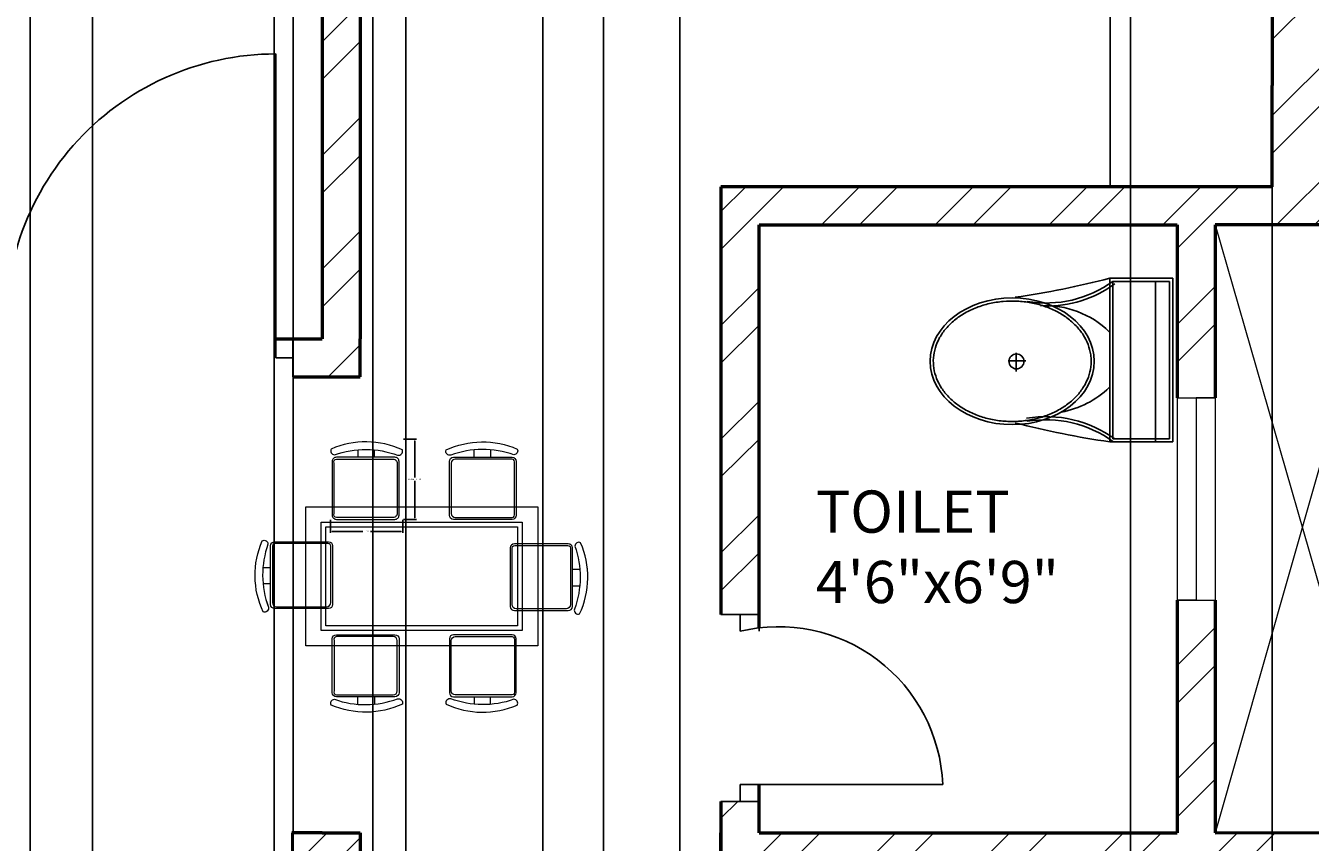
# Model space of a CAD drawing. Units: inches. Extents: x 1980 to 2738, y 1471 to 2568.
# Tile 18 of 22: x 2211 to 2363, y 2232 to 2329. Entities that reach past the tile are written whole.
import ezdxf

# ---------------------------------------------------------------- set-up
doc = ezdxf.new("R2010")
doc.units = ezdxf.units.IN
for name, color, linetype, lineweight in [('A-ANNO-DIMS', 2, 'Continuous', 18), ('A-AREA-IDEN', 7, 'Continuous', 18), ('A-DOOR', 31, 'Continuous', 25), ('A-FLOR-CASE', 8, 'Continuous', 25), ('A-FLOR-FIXT', 8, 'Continuous', 25), ('A-FLOR-OPEN', 8, 'Continuous', 18), ('A-FURN', 8, 'Continuous', 18), ('A-GLAZ', 141, 'Continuous', 18), ('A-WALL', 7, 'Continuous', 50)]:
    doc.layers.add(name, color=color, linetype=linetype, lineweight=lineweight)
doc.layers.add('A-WALL-PATT', color=9, linetype='Continuous', lineweight=13, true_color=0xd19cc7)
doc.styles.get("Standard").update_dxf_attribs({"font": 'arial.ttf'})
doc.dimstyles.get("Standard").update_dxf_attribs({"dimtxt": 0.18, "dimasz": 0.18, "dimexe": 0.18, "dimexo": 0.0625, "dimgap": 0.09, "dimtad": 0, "dimtih": 1, "dimtoh": 1, "dimdec": 4, "dimzin": 0, "dimdsep": 46, "dimtxsty": 'Standard', "dimcen": 0.09, "dimadec": 0, "dimazin": 0, "dimtfac": 1, "dimtdec": 4, "dimtofl": 0, "dimtmove": 0, "dimatfit": 3, "dimfxl": 1, "dimtolj": 1, "dimtzin": 0, "dimarcsym": 0})

# ---------------------------------------------------------------- blocks, each defined once
blk = doc.blocks.new('A$C31115884')
for p, q in [((283.1, 497.7), (223.4, 497.7)), ((257.5, 466.4), (257.5, 523.2)), ((0, 200), (0, 0)), ((520, 200), (0, 200)), ((10, 190), (10, 10)), ((510, 190), (10, 190)), ((510, 10), (510, 190)), ((520, 0), (520, 200)), ((510, 54.5), (0, 54.5)), ((10, 10), (510, 10)), ((0, 0), (520, 0))]:
    blk.add_line(p, q)
blk.add_circle((255.6, 496.4), 23.6)
for centre, radius, start, end in [((2777.7, -204.6), 2807, 165.4549, 171.7133), ((3237, 905), 2807, 188.2867, 194.5451), ((-294.5, 403.3), 364.7, 324.2091, 9.3499), ((-294.5, 403.3), 374.7, 324.2091, 9.3499), ((805.8, 403.3), 364.7, 170.6501, 215.7909), ((139.5, 406.2), 293.5, 315.8436, 2.6563), ((805.8, 403.3), 374.7, 179.2036, 215.7909), ((383.6, 406.2), 293.5, 190.2774, 224.1564)]:
    blk.add_arc(centre, radius, start, end)
blk.add_ellipse((256.2, 509.9), major_axis=(0, -260.7), ratio=0.772727)
blk.add_open_spline([(256.2, 259.2), (263.1, 259.2), (270, 259.7), (287.8, 262.3), (298.7, 265.1), (319.9, 273.1), (330.2, 278.4), (350.1, 291.1), (359.7, 298.7), (377.7, 315.9), (386.2, 325.5), (401.7, 346.6), (408.8, 358.1), (421.3, 382.5), (426.8, 395.5), (435.9, 422.4), (439.5, 436.4), (444.8, 465.1), (446.5, 479.7), (447.9, 509.2), (447.6, 524), (445, 553.3), (442.7, 567.8), (436.3, 596), (432.1, 609.7), (421.9, 636), (416, 648.6), (402.5, 672.1), (395, 683), (378.6, 703), (369.8, 712.1), (351.1, 728), (341.3, 734.8), (320.9, 746.2), (310.4, 750.7), (288.9, 757.3), (278, 759.4), (256, 761), (245, 760.6), (223.1, 757.2), (212.3, 754.3), (191.1, 746.1), (180.8, 740.7), (160.9, 727.8), (151.4, 720.1), (133.5, 702.7), (125.1, 693), (109.6, 671.7), (102.6, 660.2), (90.2, 635.7), (84.9, 622.7), (76, 595.6), (72.4, 581.6), (67.2, 552.9), (65.6, 538.2), (64.4, 508.8), (64.8, 494), (67.5, 464.7), (69.9, 450.2), (76.6, 422), (80.8, 408.3), (91.1, 382.2), (97.2, 369.7), (110.8, 346.3), (118.4, 335.4), (134.8, 315.6), (143.7, 306.7), (162.4, 290.9), (172.3, 284.2), (192.8, 273), (203.3, 268.6), (224.8, 262.2), (235.8, 260.2), (249.9, 259.3), (253, 259.2), (256.2, 259.2)], degree=3, knots=[0, 0, 0, 0, 0.110105, 0.110105, 0.285049, 0.285049, 0.459994, 0.459994, 0.634938, 0.634938, 0.809882, 0.809882, 0.984827, 0.984827, 1.159771, 1.159771, 1.334715, 1.334715, 1.50966, 1.50966, 1.684604, 1.684604, 1.859549, 1.859549, 2.034493, 2.034493, 2.209437, 2.209437, 2.384382, 2.384382, 2.559326, 2.559326, 2.73427, 2.73427, 2.909215, 2.909215, 3.084159, 3.084159, 3.259103, 3.259103, 3.434048, 3.434048, 3.608992, 3.608992, 3.783936, 3.783936, 3.958881, 3.958881, 4.133825, 4.133825, 4.30877, 4.30877, 4.483714, 4.483714, 4.658658, 4.658658, 4.833603, 4.833603, 5.008547, 5.008547, 5.183491, 5.183491, 5.358436, 5.358436, 5.53338, 5.53338, 5.708324, 5.708324, 5.883269, 5.883269, 6.058213, 6.058213, 6.233158, 6.233158, 6.283185, 6.283185, 6.283185, 6.283185])
blk = doc.blocks.new('TABLE-DINING-RECT')
for points in [[(0, 16.47), (27.45, 16.47), (27.45, 0), (0, 0)], [(0, 16.47), (27.45, 16.47), (27.45, 0), (0, 0)], [(1.83, 14.64), (25.62, 14.64), (25.62, 1.83), (1.83, 1.83)], [(1.83, 14.64), (25.62, 14.64), (25.62, 1.83), (1.83, 1.83)], [(2.38, 14.09), (25.07, 14.09), (25.07, 2.38), (2.38, 2.38)], [(2.38, 14.09), (25.07, 14.09), (25.07, 2.38), (2.38, 2.38)]]:
    blk.add_lwpolyline(points, close=True)
blk = doc.blocks.new('CHAIR-DINING')
for points in [[(0.45, 7.65, -0.175809), (7.92, 7.6, 0.578392), (8.49, 8.22, 0.214524), (0.05, 8.33, 0.552014), (0.45, 7.65, -0.065079)], [(0.45, 7.65, -0.175809), (7.92, 7.6, 0.578392), (8.49, 8.22, 0.214524), (0.05, 8.33, 0.552014), (0.45, 7.65, -0.065079)], [(5.17, 7.35), (5.17, 8.23, -0.064759)], [(5.17, 7.35), (5.17, 8.23, -0.064759)], [(7.61, 7.35), (0.67, 7.35, 0.414214), (0.18, 6.87), (0.18, 0.49, 0.414214), (0.67, 0), (7.61, 0, 0.414214), (8.09, 0.49), (8.09, 6.87, 0.414214), (7.61, 7.35)], [(7.61, 7.35), (0.67, 7.35, 0.414214), (0.18, 6.87), (0.18, 0.49, 0.414214), (0.67, 0), (7.61, 0, 0.414214), (8.09, 0.49), (8.09, 6.87, 0.414214), (7.61, 7.35)]]:
    blk.add_lwpolyline(points, format="xyb")
blk.add_lwpolyline([(3.23, 8.25), (3.23, 7.35)])
blk.add_lwpolyline([(3.23, 8.25), (3.23, 7.35)])
blk.add_lwpolyline([(0.67, 7.13), (7.39, 7.13, -0.414214), (7.87, 6.65), (7.87, 0.7, -0.414214), (7.39, 0.22), (0.67, 0.22, -0.512069), (0.4, 0.7), (0.4, 6.65, -0.512069)], format="xyb", close=True)
blk.add_lwpolyline([(0.67, 7.13), (7.39, 7.13, -0.414214), (7.87, 6.65), (7.87, 0.7, -0.414214), (7.39, 0.22), (0.67, 0.22, -0.512069), (0.4, 0.7), (0.4, 6.65, -0.512069)], format="xyb", close=True)
blk = doc.blocks.new('WIN-24IN-PARTITION')
for p, q in [((0, 24), (4.5, 24)), ((0, 24), (0, 0)), ((4.5, 24), (2.25, 24)), ((2.25, 24), (2.25, 0)), ((4.5, 24), (4.5, 0)), ((2.25, 0), (0, 0)), ((0, 0), (4.5, 0))]:
    blk.add_line(p, q)
blk = doc.blocks.new('SHAFT-OPENING-MARK')
for p, q in [((20.51, 72), (0, 0)), ((0, 72), (20.71, 0.06))]:
    blk.add_line(p, q)
blk = doc.blocks.new('*D27')
at = {"layer": 'A-ANNO-DIMS', "color": 0, "lineweight": -2, "transparency": 16777216}
for p, q in [((2255.71, 2279.83), (2257.25, 2279.83)), ((2257.07, 2279.65), (2257.07, 2275.27)), ((2257.07, 2270.51), (2257.07, 2274.9)), ((2255.71, 2270.33), (2257.25, 2270.33))]:
    blk.add_line(p, q, dxfattribs=at)
at = {"layer": 'A-ANNO-DIMS', "color": 0, "transparency": 16777216}
for points in [[(2257.04, 2279.65), (2257.1, 2279.65), (2257.07, 2279.83)], [(2257.04, 2270.51), (2257.1, 2270.51), (2257.07, 2270.33)]]:
    blk.add_solid(points, dxfattribs=at)
at = {"layer": 'Defpoints', "color": 0, "transparency": 16777216}
for p in [(2255.64, 2279.83), (2257.07, 2279.83), (2255.64, 2270.33)]:
    blk.add_point(p, dxfattribs=at)
at = {"layer": 'A-ANNO-DIMS', "color": 0, "transparency": 16777216, "insert": (2257.07, 2275.08), "char_height": 0.18, "attachment_point": 5}
blk.add_mtext('\\A1;CHAIR 10 TYP.', dxfattribs=at)
blk = doc.blocks.new('*D28')
at = {"layer": 'A-ANNO-DIMS', "color": 0, "lineweight": -2, "transparency": 16777216}
for p, q in [((2247.08, 2270.27), (2247.08, 2268.73)), ((2255.64, 2270.27), (2255.64, 2268.73)), ((2247.26, 2268.91), (2250.9, 2268.91)), ((2255.46, 2268.91), (2251.82, 2268.91))]:
    blk.add_line(p, q, dxfattribs=at)
at = {"layer": 'A-ANNO-DIMS', "color": 0, "transparency": 16777216}
for points in [[(2247.26, 2268.94), (2247.26, 2268.88), (2247.08, 2268.91)], [(2255.46, 2268.94), (2255.46, 2268.88), (2255.64, 2268.91)]]:
    blk.add_solid(points, dxfattribs=at)
at = {"layer": 'Defpoints', "color": 0, "transparency": 16777216}
for p in [(2247.08, 2270.33), (2255.64, 2270.33), (2255.64, 2268.91)]:
    blk.add_point(p, dxfattribs=at)
at = {"layer": 'A-ANNO-DIMS', "color": 0, "transparency": 16777216, "insert": (2251.36, 2268.91), "char_height": 0.18, "attachment_point": 5}
blk.add_mtext('\\A1;9 TYP.', dxfattribs=at)
blk = doc.blocks.new('*D35')
at = {"layer": 'A-ANNO-DIMS', "color": 0, "lineweight": -2, "transparency": 16777216}
for p, q in [((2081.08, 2291.77), (2081.08, 2507.54)), ((2081.26, 2507.36), (2362.79, 2507.36)), ((2644.9, 2507.36), (2363.37, 2507.36)), ((2645.08, 2291.77), (2645.08, 2507.54))]:
    blk.add_line(p, q, dxfattribs=at)
at = {"layer": 'A-ANNO-DIMS', "color": 0, "transparency": 16777216}
for points in [[(2081.26, 2507.39), (2081.26, 2507.33), (2081.08, 2507.36)], [(2644.9, 2507.39), (2644.9, 2507.33), (2645.08, 2507.36)]]:
    blk.add_solid(points, dxfattribs=at)
at = {"layer": 'Defpoints', "color": 0, "transparency": 16777216}
for p in [(2645.08, 2507.36), (2081.08, 2291.71), (2645.08, 2291.71)]:
    blk.add_point(p, dxfattribs=at)
at = {"layer": 'A-ANNO-DIMS', "color": 0, "transparency": 16777216, "insert": (2363.08, 2507.36), "char_height": 0.18, "attachment_point": 5}
blk.add_mtext('\\A1;564', dxfattribs=at)
blk = doc.blocks.new('*D44')
at = {"layer": 'A-ANNO-DIMS', "color": 0, "lineweight": -2, "transparency": 16777216}
for p, q in [((2218.88, 1694.77), (2218.88, 2507.54)), ((2219.06, 2507.36), (2229.18, 2507.36)), ((2240.22, 2507.36), (2230.11, 2507.36)), ((2240.4, 1694.77), (2240.4, 2507.54))]:
    blk.add_line(p, q, dxfattribs=at)
at = {"layer": 'A-ANNO-DIMS', "color": 0, "transparency": 16777216}
for points in [[(2219.06, 2507.39), (2219.06, 2507.33), (2218.88, 2507.36)], [(2240.22, 2507.39), (2240.22, 2507.33), (2240.4, 2507.36)]]:
    blk.add_solid(points, dxfattribs=at)
at = {"layer": 'Defpoints', "color": 0, "transparency": 16777216}
for p in [(2240.4, 2507.36), (2218.88, 1694.71), (2240.4, 1694.71)]:
    blk.add_point(p, dxfattribs=at)
at = {"layer": 'A-ANNO-DIMS', "color": 0, "transparency": 16777216, "insert": (2229.64, 2507.36), "char_height": 0.18, "attachment_point": 5}
blk.add_mtext('\\A1;21.525', dxfattribs=at)
blk = doc.blocks.new('*D45')
at = {"layer": 'A-ANNO-DIMS', "color": 0, "lineweight": -2, "transparency": 16777216}
for p, q in [((2255.99, 1694.77), (2255.99, 2507.54)), ((2256.17, 2507.36), (2267.22, 2507.36)), ((2279.21, 2507.36), (2268.15, 2507.36)), ((2279.39, 1694.77), (2279.39, 2507.54))]:
    blk.add_line(p, q, dxfattribs=at)
at = {"layer": 'A-ANNO-DIMS', "color": 0, "transparency": 16777216}
for points in [[(2256.17, 2507.39), (2256.17, 2507.33), (2255.99, 2507.36)], [(2279.21, 2507.39), (2279.21, 2507.33), (2279.39, 2507.36)]]:
    blk.add_solid(points, dxfattribs=at)
at = {"layer": 'Defpoints', "color": 0, "transparency": 16777216}
for p in [(2279.39, 2507.36), (2255.99, 1694.71), (2279.39, 1694.71)]:
    blk.add_point(p, dxfattribs=at)
at = {"layer": 'A-ANNO-DIMS', "color": 0, "transparency": 16777216, "insert": (2267.69, 2507.36), "char_height": 0.18, "attachment_point": 5}
blk.add_mtext('\\A1;23.407', dxfattribs=at)
blk = doc.blocks.new('*D46')
at = {"layer": 'A-ANNO-DIMS', "color": 0, "lineweight": -2, "transparency": 16777216}
for p, q in [((2211.52, 1814.77), (2211.52, 2507.54)), ((2211.7, 2507.36), (2226.69, 2507.36)), ((2242.46, 2507.36), (2227.48, 2507.36)), ((2242.64, 1814.77), (2242.64, 2507.54))]:
    blk.add_line(p, q, dxfattribs=at)
at = {"layer": 'A-ANNO-DIMS', "color": 0, "transparency": 16777216}
for points in [[(2211.7, 2507.39), (2211.7, 2507.33), (2211.52, 2507.36)], [(2242.46, 2507.39), (2242.46, 2507.33), (2242.64, 2507.36)]]:
    blk.add_solid(points, dxfattribs=at)
at = {"layer": 'Defpoints', "color": 0, "transparency": 16777216}
for p in [(2242.64, 2507.36), (2211.52, 1814.71), (2242.64, 1814.71)]:
    blk.add_point(p, dxfattribs=at)
at = {"layer": 'A-ANNO-DIMS', "color": 0, "transparency": 16777216, "insert": (2227.08, 2507.36), "char_height": 0.18, "attachment_point": 5}
blk.add_mtext('\\A1;31.12', dxfattribs=at)
blk = doc.blocks.new('*D50')
at = {"layer": 'A-ANNO-DIMS', "color": 0, "lineweight": -2, "transparency": 16777216}
for p, q in [((2288.43, 1708.09), (2288.43, 2507.54)), ((2288.61, 2507.36), (2314.71, 2507.36)), ((2341.6, 2507.36), (2315.5, 2507.36)), ((2341.78, 1708.09), (2341.78, 2507.54))]:
    blk.add_line(p, q, dxfattribs=at)
at = {"layer": 'A-ANNO-DIMS', "color": 0, "transparency": 16777216}
for points in [[(2288.61, 2507.39), (2288.61, 2507.33), (2288.43, 2507.36)], [(2341.6, 2507.39), (2341.6, 2507.33), (2341.78, 2507.36)]]:
    blk.add_solid(points, dxfattribs=at)
at = {"layer": 'Defpoints', "color": 0, "transparency": 16777216}
for p in [(2341.78, 2507.36), (2288.43, 1708.03), (2341.78, 1708.03)]:
    blk.add_point(p, dxfattribs=at)
at = {"layer": 'A-ANNO-DIMS', "color": 0, "transparency": 16777216, "insert": (2315.11, 2507.36), "char_height": 0.18, "attachment_point": 5}
blk.add_mtext('\\A1;53.34', dxfattribs=at)
blk = doc.blocks.new('*D51')
at = {"layer": 'A-ANNO-DIMS', "color": 0, "lineweight": -2, "transparency": 16777216}
for p, q in [((2341.78, 1708.09), (2341.78, 2507.54)), ((2341.96, 2507.36), (2349.72, 2507.36)), ((2358.4, 2507.36), (2350.63, 2507.36)), ((2358.58, 1694.77), (2358.58, 2507.54))]:
    blk.add_line(p, q, dxfattribs=at)
at = {"layer": 'A-ANNO-DIMS', "color": 0, "transparency": 16777216}
for points in [[(2341.96, 2507.39), (2341.96, 2507.33), (2341.78, 2507.36)], [(2358.4, 2507.39), (2358.4, 2507.33), (2358.58, 2507.36)]]:
    blk.add_solid(points, dxfattribs=at)
at = {"layer": 'Defpoints', "color": 0, "transparency": 16777216}
for p in [(2358.58, 2507.36), (2341.78, 1708.03), (2358.58, 1694.71)]:
    blk.add_point(p, dxfattribs=at)
at = {"layer": 'A-ANNO-DIMS', "color": 0, "transparency": 16777216, "insert": (2350.18, 2507.36), "char_height": 0.18, "attachment_point": 5}
blk.add_mtext('\\A1;16.807', dxfattribs=at)
blk = doc.blocks.new('*D54')
at = {"layer": 'A-ANNO-DIMS', "color": 0, "lineweight": -2, "transparency": 16777216}
for p, q in [((2252.1, 1949.01), (2252.1, 2507.54)), ((2252.28, 2507.36), (2261.78, 2507.36)), ((2272.03, 2507.36), (2262.53, 2507.36)), ((2272.21, 1949.01), (2272.21, 2507.54))]:
    blk.add_line(p, q, dxfattribs=at)
at = {"layer": 'A-ANNO-DIMS', "color": 0, "transparency": 16777216}
for points in [[(2252.28, 2507.39), (2252.28, 2507.33), (2252.1, 2507.36)], [(2272.03, 2507.39), (2272.03, 2507.33), (2272.21, 2507.36)]]:
    blk.add_solid(points, dxfattribs=at)
at = {"layer": 'Defpoints', "color": 0, "transparency": 16777216}
for p in [(2272.21, 2507.36), (2252.1, 1948.95), (2272.21, 1948.95)]:
    blk.add_point(p, dxfattribs=at)
at = {"layer": 'A-ANNO-DIMS', "color": 0, "transparency": 16777216, "insert": (2262.16, 2507.36), "char_height": 0.18, "attachment_point": 5}
blk.add_mtext('\\A1;20.11', dxfattribs=at)

msp = doc.modelspace()

# ---------------------------------------------------------------- hatches: boundary and pattern name
at = {"layer": 'A-WALL-PATT'}
h = msp.add_hatch(dxfattribs=at)
h.set_pattern_fill('ANSI32', color=256)
h.paths.add_polyline_path([(2257.5661, 2416.2064), (2257.5661, 2420.7064), (2250.5833, 2420.7064), (2250.5833, 2462.7064), (2246.0833, 2462.7064), (2246.0833, 2420.7064), (2237.0791, 2420.7064), (2237.0791, 2411.7064), (2246.0833, 2411.7064), (2246.0833, 2291.7064), (2242.6109, 2291.7064), (2242.6109, 2287.2064), (2246.0833, 2287.2064), (2250.5833, 2287.2064), (2250.5833, 2291.7064), (2250.5833, 2411.7064), (2257.5661, 2411.7064)])
h.paths.add_polyline_path([(2387.0396, 2416.2064), (2387.0396, 2420.7064), (2367.5833, 2420.7064), (2367.5833, 2462.7064), (2358.5833, 2462.7064), (2358.5833, 2420.7064), (2329.3087, 2420.7064), (2329.3087, 2411.7064), (2358.5833, 2411.7064), (2358.5833, 2321.7275), (2358.5833, 2309.7064), (2347.3089, 2309.7064), (2293.3089, 2309.7064), (2293.3089, 2259.0771), (2297.8089, 2259.0771), (2297.8089, 2305.2064), (2347.3089, 2305.2064), (2347.3089, 2284.7412), (2351.8089, 2284.7412), (2351.8089, 2305.2064), (2372.3188, 2305.2064), (2372.3761, 2284.3899), (2377.0295, 2284.3899), (2377.0295, 2299.3058), (2377.0295, 2305.2064), (2426.5295, 2305.2064), (2426.5295, 2257.5573), (2431.0295, 2257.5573), (2431.0295, 2309.7064), (2377.0295, 2309.7064), (2367.5833, 2309.7064), (2367.5833, 2321.7275), (2367.5833, 2411.7064), (2387.0396, 2411.7064)])
h.paths.add_polyline_path([(2448.5267, 2416.2064), (2448.5267, 2420.7064), (2423.0396, 2420.7064), (2423.0396, 2411.7064), (2448.5267, 2411.7064)])
h.paths.add_polyline_path([(2130.9128, 2416.2064), (2130.9128, 2420.7064), (2105.0833, 2420.7064), (2105.0833, 2386.6942), (2114.0833, 2386.6942), (2114.0833, 2411.7064), (2130.9128, 2411.7064)])
h.paths.add_polyline_path([(2212.9478, 2420.7064), (2190.9128, 2420.7064), (2190.9128, 2411.7064), (2212.9478, 2411.7064), (2212.9478, 2416.2064)])
h.paths.add_polyline_path([(2114.0833, 2326.6942), (2105.0833, 2326.6942), (2105.0833, 2291.7064), (2081.0833, 2291.7064), (2081.0833, 2287.2064), (2105.0833, 2287.2064), (2105.0833, 2276.1935), (2114.0833, 2276.1935), (2114.0833, 2287.2064), (2166.3825, 2287.2064), (2166.3825, 2289.4564), (2166.3825, 2291.7064), (2114.0833, 2291.7064)])
h.paths.add_polyline_path([(2114.0833, 2252.1935), (2105.0833, 2252.1935), (2105.0833, 2233.2064), (2081.0833, 2233.2064), (2081.0833, 2228.7064), (2105.0833, 2228.7064), (2105.0833, 2213.4478), (2114.0833, 2213.4478), (2114.0833, 2228.7064), (2195.0833, 2228.7064), (2199.5833, 2228.7064), (2208.4455, 2228.7064), (2208.4455, 2230.9564), (2208.4455, 2233.2064), (2199.5833, 2233.2064), (2199.5833, 2287.2064), (2206.8904, 2287.2064), (2206.8904, 2289.4564), (2206.8904, 2291.7064), (2189.446, 2291.7064), (2189.446, 2289.4564), (2189.446, 2287.2064), (2195.0833, 2287.2064), (2195.0833, 2233.2064), (2114.0833, 2233.2064)])
h.paths.add_polyline_path([(2114.0833, 2153.4478), (2109.5833, 2153.4478), (2105.0833, 2153.4478), (2105.0833, 2135.2374), (2114.0833, 2135.2374)], flags=17)
h.paths.add_polyline_path([(2135.9619, 2095.4081), (2140.1805, 2095.4081), (2140.1805, 2104.2064), (2114.0833, 2104.2064), (2114.0833, 2110.3997), (2109.5833, 2110.3997), (2105.0833, 2110.3997), (2105.0833, 2104.2064), (2081.0833, 2104.2064), (2081.0833, 2099.7064), (2105.0833, 2099.7064), (2127.5416, 2099.8532), (2127.5416, 2056.9393), (2136.2133, 2056.9393)], flags=17)
h.paths.add_polyline_path([(2255.4895, 2104.2064), (2250.5833, 2104.2064), (2250.5833, 2233.2064), (2246.0833, 2233.2064), (2242.4941, 2233.2064), (2242.4941, 2228.7064), (2246.0833, 2228.7064), (2246.0833, 2104.2064), (2163.6825, 2104.2064), (2163.6825, 2099.8072), (2163.6825, 2095.4081), (2191.4325, 2095.4081), (2191.4325, 2011.2064), (2186.0833, 2011.2064), (2136.5143, 2010.8824), (2136.3702, 2032.9403), (2131.9559, 2032.9115), (2127.5416, 2032.8826), (2127.5416, 2006.7064), (2105.0833, 2006.7064), (2081.0833, 2006.7064), (2081.0833, 2002.2064), (2105.0833, 2002.2064), (2105.0833, 1995.9329), (2114.0833, 1995.9329), (2114.0833, 2002.2064), (2246.0833, 2002.2064), (2246.0833, 1877.7064), (2242.1358, 1877.7064), (2242.1358, 1873.2064), (2250.5833, 1873.2064), (2250.5833, 2002.2064), (2255.3335, 2002.2064), (2255.3335, 2011.2064), (2195.9325, 2011.2064), (2195.9325, 2095.2064), (2255.4895, 2095.2064), (2255.4895, 2099.5471)])
h.paths.add_polyline_path([(2199.5833, 1873.2064), (2209.827, 1873.2064), (2209.827, 1875.4564), (2209.827, 1877.7064), (2114.0833, 1877.7064), (2114.0833, 1890.0968), (2105.0833, 1890.0968), (2105.0833, 1877.7064), (2081.0833, 1877.7064), (2081.0833, 1873.2064), (2105.0833, 1873.2064), (2105.0833, 1857.7279), (2114.0833, 1857.7279), (2114.0833, 1873.2064), (2195.0833, 1873.2064), (2195.0833, 1819.2064), (2190.298, 1819.2064), (2190.298, 1814.7064), (2209.8976, 1814.7064), (2209.8976, 1816.9564), (2209.8976, 1819.2064), (2199.5833, 1819.2064)])
h.paths.add_polyline_path([(2114.0833, 1814.7064), (2166.2538, 1814.7064), (2166.2538, 1816.9564), (2166.2538, 1819.2064), (2114.0833, 1819.2064), (2114.0833, 1833.7279), (2109.5833, 1833.7279), (2105.0833, 1833.7279), (2105.0833, 1819.2064), (2081.0833, 1819.2064), (2081.0833, 1814.7064), (2105.0833, 1814.7064), (2105.0833, 1782.5516), (2114.0833, 1782.5516)])
h.paths.add_polyline_path([(2114.0833, 1722.5516), (2109.5833, 1722.5516), (2105.0833, 1722.5516), (2105.0833, 1685.7064), (2124.5104, 1685.7064), (2124.5104, 1690.2064), (2124.5104, 1694.7064), (2114.0833, 1694.7064)])
h.paths.add_polyline_path([(2218.8787, 1694.7064), (2184.5104, 1694.7064), (2184.5104, 1685.7064), (2218.8787, 1685.7064), (2218.8787, 1690.2064)])
h.paths.add_polyline_path([(2250.5833, 1819.2064), (2242.6431, 1819.2064), (2242.6431, 1816.9564), (2242.6431, 1814.7064), (2246.0833, 1814.7064), (2246.0833, 1694.7064), (2240.4035, 1694.7064), (2240.4035, 1690.2064), (2240.4035, 1685.7064), (2246.0833, 1685.7064), (2246.0833, 1643.7064), (2250.5833, 1643.7064), (2250.5833, 1685.7064), (2255.9859, 1685.7064), (2255.9859, 1690.2064), (2255.9859, 1694.7064), (2250.5833, 1694.7064)])
h.paths.add_polyline_path([(2297.4764, 1694.7064), (2279.3934, 1694.7064), (2279.3934, 1690.2064), (2279.3934, 1685.7064), (2297.4764, 1685.7064), (2297.4764, 1690.2064)])
h.paths.add_polyline_path([(2377.1596, 1694.7064), (2367.5833, 1694.7064), (2367.5833, 1787.7064), (2431.0295, 1787.7064), (2431.0295, 1792.2064), (2431.0295, 1849.4149), (2428.7795, 1849.4149), (2426.5295, 1849.4149), (2426.5295, 1792.2064), (2421.5833, 1792.2064), (2367.5833, 1792.2064), (2297.8089, 1792.2064), (2297.8089, 1850.2946), (2295.5589, 1850.2946), (2293.3089, 1850.2946), (2293.3089, 1792.2064), (2293.3089, 1787.7064), (2297.8089, 1787.7064), (2358.5833, 1787.7064), (2358.5833, 1694.7064), (2333.4764, 1694.7064), (2333.4764, 1685.7064), (2358.5833, 1685.7064), (2358.5833, 1643.7064), (2367.5833, 1643.7064), (2367.5833, 1685.7064), (2377.1596, 1685.7064)])
h.paths.add_polyline_path([(2442.4912, 1694.7064), (2413.1596, 1694.7064), (2413.1596, 1685.7064), (2442.4912, 1685.7064)])
h.paths.add_polyline_path([(2480.0833, 1814.7064), (2483.4816, 1814.7064), (2483.4816, 1817.9384), (2483.4816, 1819.2064), (2475.5833, 1819.2064), (2475.5833, 1694.7064), (2470.7283, 1694.7064), (2470.7283, 1685.7064), (2475.5833, 1685.7064), (2475.5833, 1643.7064), (2480.0833, 1643.7064), (2480.0833, 1685.7064), (2486.3293, 1685.7064), (2486.3293, 1690.2064), (2486.3293, 1694.7064), (2480.0833, 1694.7064)])
h.paths.add_polyline_path([(2621.0833, 1721.7349), (2612.0833, 1721.7349), (2612.0833, 1694.7064), (2586.1453, 1694.7064), (2586.1453, 1685.7064), (2621.0833, 1685.7064)])
h.paths.add_polyline_path([(2526.1453, 1690.2064), (2526.1453, 1694.7064), (2511.584, 1694.7064), (2511.584, 1690.2064), (2511.584, 1685.7064), (2526.1453, 1685.7064)])
h.paths.add_polyline_path([(2645.0833, 1819.2064), (2621.0833, 1819.2064), (2621.0833, 1835.8527), (2616.5833, 1835.8527), (2612.0833, 1835.8527), (2612.0833, 1819.2064), (2560.2541, 1819.2064), (2560.2541, 1814.7064), (2612.0833, 1814.7064), (2612.0833, 1781.7349), (2621.0833, 1781.7349), (2621.0833, 1814.7064), (2645.0833, 1814.7064)])
h.paths.add_polyline_path([(2645.0833, 1877.7064), (2621.0833, 1877.7064), (2621.0833, 1886.4375), (2612.0833, 1886.4375), (2612.0833, 1877.7064), (2517.1032, 1877.7064), (2517.1032, 1875.4564), (2517.1032, 1873.2064), (2526.5833, 1873.2064), (2526.5833, 1819.2064), (2516.6454, 1819.2064), (2516.6454, 1816.9564), (2516.6454, 1814.7064), (2536.4445, 1814.7064), (2536.4445, 1816.9564), (2536.4445, 1819.2064), (2531.0833, 1819.2064), (2531.0833, 1873.2064), (2612.0833, 1873.2064), (2612.0833, 1859.8527), (2621.0833, 1859.8527), (2621.0833, 1873.2064), (2645.0833, 1873.2064)])
h.paths.add_polyline_path([(2645.0833, 2006.7064), (2621.0833, 2006.7064), (2588.5085, 2006.7064), (2588.5085, 2052.9125), (2579.9045, 2052.9125), (2579.9045, 2011.2064), (2519.9045, 2011.2064), (2519.9045, 2095.2064), (2553.1204, 2095.2064), (2553.1204, 2104.2064), (2480.0833, 2104.2064), (2480.0833, 2228.7064), (2484.3832, 2228.7064), (2484.3832, 2230.9564), (2484.3832, 2233.2064), (2475.5833, 2233.2064), (2475.5833, 2104.2064), (2463.1308, 2104.2064), (2463.1308, 2095.2064), (2501.2463, 2095.2064), (2510.9045, 2095.2064), (2515.4045, 2095.2064), (2515.4045, 2011.2064), (2510.9045, 2011.2064), (2501.2463, 2011.2064), (2462.5957, 2011.2064), (2462.5957, 2002.2064), (2475.5833, 2002.2064), (2475.5833, 1873.2064), (2483.6146, 1873.2064), (2483.6146, 1875.4564), (2483.6146, 1877.7064), (2480.0833, 1877.7064), (2480.0833, 2002.2064), (2612.0833, 2002.2064), (2612.0833, 1996.309), (2621.0833, 1996.309), (2621.0833, 2002.2064), (2645.0833, 2002.2064)])
h.paths.add_polyline_path([(2588.5085, 2099.7277), (2621.0833, 2099.7277), (2645.0833, 2099.7064), (2645.0833, 2104.2064), (2621.0833, 2104.2064), (2621.0833, 2109.0038), (2616.5833, 2109.0038), (2612.0833, 2109.0038), (2612.0833, 2104.2064), (2575.0621, 2104.2064), (2575.0621, 2099.7064), (2575.0621, 2095.2064), (2579.9045, 2095.2064), (2579.9045, 2076.9125), (2588.5085, 2076.9125)], flags=17)
h.paths.add_polyline_path([(2367.5833, 2002.2064), (2373.7228, 2002.2064), (2373.7228, 2006.7064), (2373.7228, 2011.2064), (2350.7889, 2011.2064), (2350.7889, 2006.7064), (2350.7889, 2002.2064), (2358.5833, 2002.2064), (2358.5833, 1877.7064), (2293.3089, 1877.7064), (2293.3089, 1870.4987), (2297.8089, 1870.4987), (2297.8089, 1873.2064), (2347.3089, 1873.2064), (2347.3089, 1847.2208), (2351.8089, 1847.2208), (2351.8089, 1873.2064), (2372.5295, 1873.2064), (2372.5295, 1847.8619), (2377.0295, 1847.8619), (2377.0295, 1873.2064), (2426.5295, 1873.2064), (2426.5295, 1868.7339), (2431.0295, 1868.7339), (2431.0295, 1877.7064), (2367.5833, 1877.7064)])
h.paths.add_polyline_path([(2531.0833, 2287.2064), (2534.2285, 2287.2064), (2534.2285, 2291.7064), (2516.7886, 2291.7064), (2516.7886, 2287.2064), (2526.5833, 2287.2064), (2526.5833, 2233.2064), (2517.9112, 2233.2064), (2517.9112, 2230.9564), (2517.9112, 2228.7064), (2526.5833, 2228.7064), (2531.0833, 2228.7064), (2612.0833, 2228.7064), (2612.0833, 2206.8504), (2621.0833, 2206.8504), (2621.0833, 2228.7064), (2645.0833, 2228.7064), (2645.0833, 2233.2064), (2621.0833, 2233.2064), (2621.0833, 2241.8536), (2616.5833, 2241.8536), (2612.0833, 2241.8536), (2612.0833, 2233.2064), (2531.0833, 2233.2064)])
h.paths.add_polyline_path([(2645.0833, 2291.7064), (2621.0833, 2291.7064), (2621.0833, 2323.0138), (2616.5833, 2323.0138), (2612.0833, 2323.0138), (2612.0833, 2291.7064), (2559.6852, 2291.7064), (2559.6852, 2289.4564), (2559.6852, 2287.2064), (2612.0833, 2287.2064), (2612.0833, 2265.8536), (2621.0833, 2265.8536), (2621.0833, 2287.2064), (2645.0833, 2287.2064)])
h.paths.add_polyline_path([(2621.0833, 2420.7064), (2582.8189, 2420.7064), (2582.8189, 2411.7064), (2612.0833, 2411.7064), (2612.0833, 2383.0138), (2621.0833, 2383.0138)])
h.paths.add_polyline_path([(2480.0833, 2411.7064), (2485.7342, 2411.7064), (2485.7342, 2416.2064), (2485.7342, 2420.7064), (2480.0833, 2420.7064), (2480.0833, 2462.7064), (2475.5833, 2462.7064), (2475.5833, 2420.7064), (2469.4083, 2420.7064), (2469.4083, 2411.7064), (2475.5833, 2411.7064), (2475.5833, 2291.7064), (2475.5833, 2287.2064), (2482.9195, 2287.2064), (2482.9195, 2289.4564), (2482.9195, 2291.7064), (2480.0833, 2291.7064)])
h.paths.add_polyline_path([(2367.5833, 2228.7064), (2431.0295, 2228.7064), (2431.0295, 2233.2064), (2431.0295, 2237.4203), (2428.7795, 2237.4203), (2426.5295, 2237.4203), (2426.5295, 2233.2064), (2377.0295, 2233.2064), (2377.0295, 2260.3837), (2372.4423, 2260.3837), (2372.517, 2233.2635), (2351.8089, 2233.2064), (2351.8089, 2260.7412), (2347.3089, 2260.7412), (2347.3089, 2233.2064), (2297.8089, 2233.2064), (2297.8089, 2236.9324), (2293.3089, 2236.9324), (2293.3089, 2228.7064), (2358.5833, 2228.7064), (2358.5833, 2104.2064), (2353.3665, 2104.2064), (2353.3665, 2095.2064), (2373.8869, 2095.2064), (2373.8869, 2099.7064), (2373.8869, 2104.2064), (2367.5833, 2104.2064)])
h.paths.add_polyline_path([(2321.2323, 2104.2064), (2303.4895, 2104.2064), (2303.4895, 2095.2064), (2321.2323, 2095.2064), (2321.2323, 2099.7064)], flags=0)
h.paths.add_polyline_path([(2415.1308, 2099.7064), (2415.1308, 2104.2064), (2404.81, 2104.2064), (2404.81, 2095.2064), (2415.1308, 2095.2064)], flags=17)
h.paths.add_polyline_path([(2318.6336, 2011.2064), (2303.3335, 2011.2064), (2303.3335, 2002.2064), (2318.6336, 2002.2064)], flags=0)
h.paths.add_polyline_path([(2414.5957, 2011.2064), (2406.2461, 2011.2064), (2406.2461, 2006.7064), (2406.2461, 2002.2064), (2414.5957, 2002.2064)], flags=17)

# ---------------------------------------------------------------- linework, layer by layer
at = {"layer": 'A-DOOR'}
for p, q in [((2240.6109, 2289.4564), (2240.6109, 2325.4564)), ((2242.6109, 2291.7064), (2242.6109, 2287.2064)), ((2242.6109, 2289.4564), (2240.6109, 2289.4564)), ((2242.6109, 2287.2064), (2242.6109, 2289.4564)), ((2293.3089, 2259.0771), (2297.8089, 2259.0771)), ((2295.5589, 2259.0771), (2295.5589, 2257.0771)), ((2297.8089, 2259.0771), (2297.8089, 2257.0771)), ((2295.5589, 2236.9324), (2295.5589, 2238.9324)), ((2295.5589, 2238.9324), (2319.5589, 2238.9324)), ((2297.8089, 2236.9324), (2293.3089, 2236.9324)), ((2293.3089, 2236.9324), (2293.3089, 2236.9324)), ((2293.3089, 2236.9324), (2295.5589, 2236.9324)), ((2297.8089, 2236.9324), (2297.8089, 2236.9324)), ((2242.4941, 2233.2064), (2242.4941, 2228.7064))]:
    msp.add_line(p, q, dxfattribs=at)
for centre, radius, start, end in [((2240.6109, 2293.4816), 31.9749, 90, 187.23183), ((2300.1174, 2238.1618), 19.4568, 2.269775, 103.549575)]:
    msp.add_arc(centre, radius, start, end, dxfattribs=at)
at = {"layer": 'A-FLOR-CASE'}
msp.add_line((2339.3978, 2397.4159), (2339.3978, 2309.7064), dxfattribs=at)
at = {"layer": 'A-FURN'}
for points in [[(2261.3168, 2277.927, -0.57839206), (2260.7505, 2278.5497, -0.21452438), (2269.1886, 2278.6629, -0.55201397), (2268.7922, 2277.9836, 0.1758092), (2261.3168, 2277.927)], [(2261.3168, 2277.9267, -0.57839206), (2260.7505, 2278.5494, -0.21452438), (2269.1887, 2278.6626, -0.55201397), (2268.7922, 2277.9833, 0.1758092), (2261.3168, 2277.9267)], [(2264.0716, 2277.6835), (2264.0716, 2278.5612, 0.06475861)], [(2264.0716, 2277.6833), (2264.0716, 2278.5609, 0.06475861)], [(2268.5739, 2277.6835, -0.41421356), (2269.0594, 2277.198), (2269.0594, 2270.8169, -0.41421356), (2268.5739, 2270.3313), (2261.6339, 2270.3313, -0.41421356), (2261.1484, 2270.8169), (2261.1484, 2277.198, -0.41421356), (2261.6339, 2277.6835), (2268.5739, 2277.6835)], [(2268.5739, 2277.6833, -0.41421356), (2269.0594, 2277.1977), (2269.0594, 2270.8166, -0.41421356), (2268.5739, 2270.3311), (2261.6339, 2270.3311, -0.41421356), (2261.1484, 2270.8166), (2261.1484, 2277.1977, -0.41421356), (2261.6339, 2277.6833), (2268.5739, 2277.6833)], [(2239.7272, 2259.9315, -0.57839206), (2239.1045, 2259.3652, -0.21452438), (2238.9913, 2267.8034, -0.55201397), (2239.6706, 2267.407, 0.17580937), (2239.7272, 2259.9315)], [(2239.7273, 2259.9312, -0.57839206), (2239.1045, 2259.3649, -0.21452438), (2238.9913, 2267.8031, -0.55201397), (2239.6707, 2267.4067, 0.17580937), (2239.7273, 2259.9312)], [(2239.9707, 2267.1886, -0.41421356), (2240.4562, 2267.6741), (2246.8373, 2267.6741, -0.41421356), (2247.3229, 2267.1886), (2247.3229, 2260.2487, -0.41421356), (2246.8373, 2259.7632), (2240.4562, 2259.7632, -0.41421356), (2239.9707, 2260.2487), (2239.9707, 2267.1886)], [(2239.9707, 2267.1883, -0.41421356), (2240.4562, 2267.6739), (2246.8373, 2267.6739, -0.41421356), (2247.3229, 2267.1883), (2247.3229, 2260.2484, -0.41421356), (2246.8373, 2259.7629), (2240.4562, 2259.7629, -0.41421356), (2239.9707, 2260.2484), (2239.9707, 2267.1883)], [(2275.7081, 2266.9509, 0.41421356), (2275.2226, 2267.4365), (2268.8415, 2267.4365, 0.41421356), (2268.3559, 2266.9509), (2268.3559, 2260.011, 0.41421356), (2268.8415, 2259.5255), (2275.2226, 2259.5255, 0.41421356), (2275.7081, 2260.011), (2275.7081, 2266.9509)], [(2275.7081, 2266.9507, 0.41421356), (2275.2226, 2267.4362), (2268.8415, 2267.4362, 0.41421356), (2268.3559, 2266.9507), (2268.3559, 2260.0107, 0.41421356), (2268.8415, 2259.5252), (2275.2226, 2259.5252, 0.41421356), (2275.7081, 2260.0107), (2275.7081, 2266.9507)], [(2276.0082, 2267.1693, -0.17580919), (2275.9515, 2259.6939, 0.57839206), (2276.5743, 2259.1275, 0.21452438), (2276.6875, 2267.5657, 0.55201397), (2276.0082, 2267.1693, -0.06507904)], [(2276.0082, 2267.169, -0.17580919), (2275.9516, 2259.6936, 0.57839206), (2276.5743, 2259.1272, 0.21452438), (2276.6875, 2267.5654, 0.55201397), (2276.0082, 2267.169, -0.06507904)], [(2239.9707, 2262.6863), (2239.093, 2262.6863, 0.06475861)], [(2239.9707, 2262.686), (2239.093, 2262.686, 0.06475861)], [(2275.7081, 2262.4487), (2276.5858, 2262.4487, -0.06475861)], [(2275.7081, 2262.4484), (2276.5858, 2262.4484, -0.06475861)], [(2254.7063, 2249.3178), (2247.7663, 2249.3178, -0.41421356), (2247.2808, 2249.8033), (2247.2808, 2256.1845, -0.41421356), (2247.7663, 2256.67), (2254.7063, 2256.67, -0.41421356), (2255.1918, 2256.1845), (2255.1918, 2249.8033, -0.41421356), (2254.7063, 2249.3178)], [(2254.7063, 2249.3175), (2247.7663, 2249.3175, -0.41421356), (2247.2808, 2249.803), (2247.2808, 2256.1842, -0.41421356), (2247.7663, 2256.6697), (2254.7063, 2256.6697, -0.41421356), (2255.1918, 2256.1842), (2255.1918, 2249.803, -0.41421356), (2254.7063, 2249.3175)], [(2268.5739, 2249.3178, 0.41421356), (2269.0594, 2249.8033), (2269.0594, 2256.1845, 0.41421356), (2268.5739, 2256.67), (2261.6339, 2256.67, 0.41421356), (2261.1484, 2256.1845), (2261.1484, 2249.8033, 0.41421356), (2261.6339, 2249.3178), (2268.5739, 2249.3178)], [(2268.5739, 2249.3175, 0.41421356), (2269.0594, 2249.803), (2269.0594, 2256.1842, 0.41421356), (2268.5739, 2256.6697), (2261.6339, 2256.6697, 0.41421356), (2261.1484, 2256.1842), (2261.1484, 2249.803, 0.41421356), (2261.6339, 2249.3175), (2268.5739, 2249.3175)], [(2255.0234, 2249.0744, -0.57839206), (2255.5897, 2248.4517, -0.21452438), (2247.1516, 2248.3384, -0.55201397), (2247.548, 2249.0178, 0.17580929), (2255.0234, 2249.0744)], [(2255.0234, 2249.0741, -0.57839206), (2255.5898, 2248.4514, -0.21452438), (2247.1516, 2248.3382, -0.55201397), (2247.548, 2249.0175, 0.17580929), (2255.0234, 2249.0741)], [(2252.2686, 2249.3178), (2252.2686, 2248.4401, 0.06475861)], [(2252.2686, 2249.3175), (2252.2686, 2248.4398, 0.06475861)], [(2268.7922, 2249.0178, -0.17580928), (2261.3168, 2249.0744, 0.57839206), (2260.7505, 2248.4517, 0.21452438), (2269.1886, 2248.3384, 0.55201397), (2268.7922, 2249.0178, -0.06507904)], [(2268.7922, 2249.0175, -0.17580928), (2261.3168, 2249.0741, 0.57839206), (2260.7505, 2248.4514, 0.21452438), (2269.1887, 2248.3382, 0.55201397), (2268.7922, 2249.0175, -0.06507904)], [(2264.0716, 2249.3178), (2264.0716, 2248.4401, -0.06475861)], [(2264.0716, 2249.3175), (2264.0716, 2248.4398, -0.06475861)]]:
    msp.add_lwpolyline(points, format="xyb", dxfattribs=at)
for points in [[(2266.0142, 2278.5772), (2266.0142, 2277.6835)], [(2266.0142, 2278.5769), (2266.0142, 2277.6833)], [(2239.077, 2264.6289), (2239.9707, 2264.6289)], [(2239.077, 2264.6286), (2239.9707, 2264.6286)], [(2276.6018, 2264.3913), (2275.7081, 2264.3913)], [(2276.6018, 2264.391), (2275.7081, 2264.391)], [(2250.326, 2248.4242), (2250.326, 2249.3178)], [(2250.326, 2248.4239), (2250.326, 2249.3175)], [(2266.0142, 2248.4242), (2266.0142, 2249.3178)], [(2266.0142, 2248.4239), (2266.0142, 2249.3175)]]:
    msp.add_lwpolyline(points, dxfattribs=at)
for points in [[(2268.5709, 2277.4648), (2261.8527, 2277.4648, 0.41421356), (2261.3671, 2276.9793), (2261.3671, 2271.0356, 0.41421356), (2261.8527, 2270.5501), (2268.5709, 2270.5501, 0.51206948), (2268.8407, 2271.0356), (2268.8407, 2276.9793, 0.51206948)], [(2268.5709, 2277.4645), (2261.8527, 2277.4645, 0.41421356), (2261.3672, 2276.979), (2261.3672, 2271.0353, 0.41421356), (2261.8527, 2270.5498), (2268.5709, 2270.5498, 0.51206948), (2268.8407, 2271.0353), (2268.8407, 2276.979, 0.51206948)], [(2240.1894, 2267.1857), (2240.1894, 2260.4674, 0.41421356), (2240.6749, 2259.9819), (2246.6186, 2259.9819, 0.41421356), (2247.1041, 2260.4674), (2247.1041, 2267.1857, 0.51206948), (2246.6186, 2267.4554), (2240.6749, 2267.4554, 0.51206948)], [(2240.1894, 2267.1854), (2240.1894, 2260.4671, 0.41421356), (2240.6749, 2259.9816), (2246.6186, 2259.9816, 0.41421356), (2247.1041, 2260.4671), (2247.1041, 2267.1854, 0.51206948), (2246.6186, 2267.4551), (2240.6749, 2267.4551, 0.51206948)], [(2275.4894, 2266.948), (2275.4894, 2260.2297, -0.41421356), (2275.0039, 2259.7442), (2269.0602, 2259.7442, -0.41421356), (2268.5747, 2260.2297), (2268.5747, 2266.948, -0.51206948), (2269.0602, 2267.2177), (2275.0039, 2267.2177, -0.51206948)], [(2275.4894, 2266.9477), (2275.4894, 2260.2294, -0.41421356), (2275.0039, 2259.7439), (2269.0602, 2259.7439, -0.41421356), (2268.5747, 2260.2294), (2268.5747, 2266.9477, -0.51206948), (2269.0602, 2267.2174), (2275.0039, 2267.2174, -0.51206948)], [(2247.7693, 2249.5365), (2254.4875, 2249.5365, 0.41421356), (2254.9731, 2250.0221), (2254.9731, 2255.9657, 0.41421356), (2254.4875, 2256.4513), (2247.7693, 2256.4513, 0.51206948), (2247.4995, 2255.9657), (2247.4995, 2250.0221, 0.51206948)], [(2247.7693, 2249.5362), (2254.4876, 2249.5362, 0.41421356), (2254.9731, 2250.0218), (2254.9731, 2255.9654, 0.41421356), (2254.4876, 2256.451), (2247.7693, 2256.451, 0.51206948), (2247.4996, 2255.9654), (2247.4996, 2250.0218, 0.51206948)], [(2268.5709, 2249.5365), (2261.8527, 2249.5365, -0.41421356), (2261.3671, 2250.0221), (2261.3671, 2255.9657, -0.41421356), (2261.8527, 2256.4513), (2268.5709, 2256.4513, -0.51206948), (2268.8407, 2255.9657), (2268.8407, 2250.0221, -0.51206948)], [(2268.5709, 2249.5362), (2261.8527, 2249.5362, -0.41421356), (2261.3672, 2250.0218), (2261.3672, 2255.9654, -0.41421356), (2261.8527, 2256.451), (2268.5709, 2256.451, -0.51206948), (2268.8407, 2255.9654), (2268.8407, 2250.0218, -0.51206948)]]:
    msp.add_lwpolyline(points, format="xyb", close=True, dxfattribs=at)
at = {"layer": 'A-GLAZ'}
msp.add_line((2347.3089, 2284.7412), (2347.3089, 2284.7412), dxfattribs=at)
at = {"layer": 'A-WALL'}
for p, q in [((2246.0833, 2411.7064), (2246.0833, 2291.7064)), ((2250.5833, 2411.7064), (2250.5833, 2291.7064)), ((2358.5833, 2411.7064), (2358.5833, 2321.7275)), ((2358.5833, 2321.7275), (2358.5833, 2321.7275)), ((2358.5833, 2309.7064), (2358.5833, 2321.7275)), ((2347.3089, 2309.7064), (2293.3089, 2309.7064)), ((2293.3089, 2309.7064), (2293.3089, 2259.0771)), ((2358.5833, 2309.7064), (2347.3089, 2309.7064)), ((2297.8089, 2305.2064), (2347.3089, 2305.2064)), ((2297.8089, 2257.4812), (2297.8089, 2305.2064)), ((2347.3089, 2305.2064), (2347.3089, 2284.7412)), ((2372.3188, 2305.2064), (2351.8089, 2305.2064)), ((2351.8089, 2305.2064), (2351.8089, 2284.7412)), ((2240.6109, 2291.7064), (2246.0833, 2291.7064)), ((2250.5833, 2287.2064), (2250.5833, 2291.7064)), ((2242.6109, 2287.2064), (2246.0833, 2287.2064)), ((2246.0833, 2287.2064), (2250.5833, 2287.2064)), ((2347.3089, 2260.7412), (2347.3089, 2233.2064)), ((2351.8089, 2260.7412), (2351.8089, 2233.2064)), ((2297.8089, 2233.2064), (2297.8089, 2238.9324)), ((2293.3089, 2236.9324), (2293.3089, 2228.7064)), ((2246.0833, 2233.2064), (2242.4941, 2233.2064)), ((2246.0833, 2233.2064), (2250.5833, 2233.2064)), ((2250.5833, 2233.2064), (2250.5833, 2104.2064)), ((2293.3089, 2228.7064), (2293.3089, 2233.2064)), ((2297.8089, 2233.2064), (2347.3089, 2233.2064)), ((2351.8089, 2233.2064), (2372.517, 2233.2635))]:
    msp.add_line(p, q, dxfattribs=at)

# ---------------------------------------------------------------- block references
at = {"layer": 'A-FLOR-FIXT', "xscale": 0.0372717239612423, "yscale": 0.0372717239612423, "zscale": 0.0372717239612423, "rotation": 89.99999999999999}
msp.add_blockref('A$C31115884', (2346.7967, 2279.5097), dxfattribs=at)
at = {"layer": 'A-FLOR-OPEN'}
msp.add_blockref('SHAFT-OPENING-MARK', (2351.809, 2233.206), dxfattribs=at)
at = {"layer": 'A-FURN'}
for name, p in [('CHAIR-DINING', (2247.099, 2270.331)), ('TABLE-DINING-RECT', (2244.153, 2255.355))]:
    msp.add_blockref(name, p, dxfattribs=at)
at = {"layer": 'A-GLAZ'}
msp.add_blockref('WIN-24IN-PARTITION', (2347.3094, 2260.7413), dxfattribs=at)

# ---------------------------------------------------------------- texts
at = {"layer": 'A-AREA-IDEN', "insert": (2304.5314, 2273.7475), "char_height": 5, "attachment_point": 1}
msp.add_mtext_dynamic_manual_height_columns('TOILET\\P4\'6"x6\'9"', width=55.958855, gutter_width=12.5, heights=[0], dxfattribs=at)

# ---------------------------------------------------------------- dimensions: what is measured, and where the dimension line sits
at = {"layer": 'A-ANNO-DIMS'}
for base, p1, p2, override, picture, middle in [((2645.0833, 2507.3564), (2081.0833, 2291.7064), (2645.0833, 2291.7064), {"dimdec": 0, "dimlfac": 1, "dimrnd": 0, "dimzin": 0, "dimdsep": 46, "dimlunit": 2}, '*D35', (2363.0833, 2507.3564)), ((2242.6431, 2507.3564), (2211.5238, 1814.7064), (2242.6431, 1814.7064), {"dimdec": 2, "dimlfac": 1, "dimrnd": 0, "dimzin": 0, "dimdsep": 46, "dimlunit": 2}, '*D46', (2227.0835, 2507.3564)), ((2240.4035, 2507.3564), (2218.8787, 1694.7064), (2240.4035, 1694.7064), {"dimdec": 3, "dimlfac": 1, "dimrnd": 0, "dimzin": 0, "dimdsep": 46, "dimlunit": 2}, '*D44', (2229.6411, 2507.3564)), ((2272.2106, 2507.3564), (2252.1, 1948.9472), (2272.2106, 1948.9472), {"dimdec": 2, "dimlfac": 1, "dimrnd": 0, "dimzin": 0, "dimdsep": 46, "dimlunit": 2}, '*D54', (2262.1553, 2507.3564)), ((2279.39337, 2507.35642), (2255.98588, 1694.70642), (2279.39337, 1694.70642), {"dimdec": 3, "dimlfac": 1, "dimrnd": 0, "dimzin": 0, "dimdsep": 46, "dimlunit": 2}, '*D45', (2267.68962, 2507.35642)), ((2341.776, 2507.3564), (2288.4349, 1708.0291), (2341.776, 1708.0291), {"dimdec": 2, "dimlfac": 1, "dimrnd": 0, "dimzin": 0, "dimdsep": 46, "dimlunit": 2}, '*D50', (2315.1054, 2507.3564)), ((2358.5833, 2507.3564), (2341.776, 1708.0291), (2358.5833, 1694.7064), {"dimdec": 3, "dimlfac": 1, "dimrnd": 0, "dimzin": 0, "dimdsep": 46, "dimlunit": 2}, '*D51', (2350.1796, 2507.3564))]:
    dim = msp.add_linear_dim(base=base, p1=p1, p2=p2, dimstyle='Standard', override=override, dxfattribs=at)
    dim.commit()
    dim.dimension.update_dxf_attribs({"geometry": picture, "text_midpoint": middle})
dim = msp.add_linear_dim(base=(2257.0683, 2279.8337), p1=(2255.6429, 2270.3311), p2=(2255.6429, 2279.8337), angle=90, text='CHAIR <> TYP.', dimstyle='Standard', override={"dimdec": 0, "dimlfac": 1, "dimrnd": 0, "dimzin": 0, "dimdsep": 46, "dimlunit": 2}, dxfattribs=at)
dim.commit()
dim.dimension.update_dxf_attribs({"geometry": '*D27', "text_midpoint": (2257.0683, 2275.0824)})
dim = msp.add_linear_dim(base=(2255.6429, 2268.9057), p1=(2247.0777, 2270.3311), p2=(2255.6429, 2270.3311), text='<> TYP.', dimstyle='Standard', override={"dimdec": 0, "dimlfac": 1, "dimrnd": 0, "dimzin": 0, "dimdsep": 46, "dimlunit": 2}, dxfattribs=at)
dim.commit()
dim.dimension.update_dxf_attribs({"geometry": '*D28', "text_midpoint": (2251.3603, 2268.9057)})

doc.saveas('drawing.dxf')
